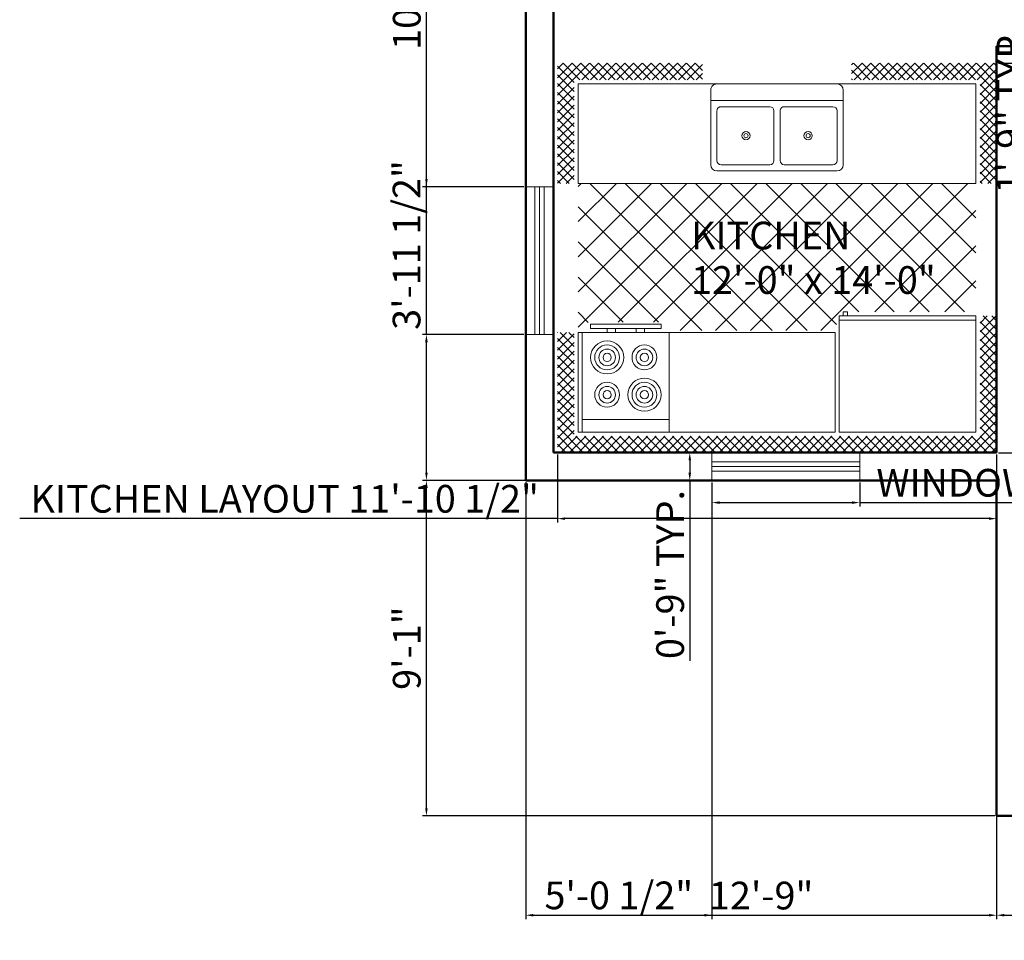
# Model space of a CAD drawing. Units: inches. Extents: x 2866 to 3545, y 873 to 1597.
# Tile 1 of 5: x 2866 to 3186, y 873 to 1172. Entities that reach past the tile are written whole.
import ezdxf

# ---------------------------------------------------------------- set-up
doc = ezdxf.new("R2010")
doc.units = ezdxf.units.IN
doc.layers.add('A-ANNO-DIMS', color=152, linetype='Continuous', lineweight=18, true_color=0x2776bb)
for name, color, linetype, lineweight in [('A-AREA-IDEN', 7, 'Continuous', 25), ('A-EQPM', 9, 'Continuous', 18), ('A-GLAZ', 4, 'Continuous', 18), ('A-WALL', 7, 'Continuous', 50)]:
    doc.layers.add(name, color=color, linetype=linetype, lineweight=lineweight)
doc.styles.get("Standard").update_dxf_attribs({"font": 'arial.ttf'})
doc.dimstyles.new('ISO-25', dxfattribs={"dimtxt": 9, "dimasz": 2.5, "dimexe": 1.25, "dimexo": 0.625, "dimtad": 1, "dimdec": 0, "dimlunit": 3, "dimtxsty": 'Standard', "dimcen": 4.5, "dimadec": 0, "dimazin": 0, "dimtfac": 1, "dimtdec": 0, "dimtmove": 0, "dimatfit": 3, "dimfxl": 1, "dimarcsym": 0})

# ---------------------------------------------------------------- blocks, each defined once
blk = doc.blocks.new('Kitchen Layout - 7 x 8 ft')
for p, q in [((-5, 81.32), (2.68, 89)), ((-5, 83.44), (0.56, 89)), ((-5, 85.56), (-1.56, 89)), ((-5, 87.68), (-3.68, 89)), ((-1, 84.97), (-5, 88.97)), ((1.09, 85), (-2.91, 89)), ((3.21, 85), (-0.79, 89)), ((0.81, 85), (4.81, 89)), ((5.34, 85), (1.34, 89)), ((2.93, 85), (6.93, 89)), ((7.46, 85), (3.46, 89)), ((5.05, 85), (9.05, 89)), ((9.58, 85), (5.58, 89)), ((7.17, 85), (11.17, 89)), ((11.7, 85), (7.7, 89)), ((9.29, 85), (13.29, 89)), ((13.82, 85), (9.82, 89)), ((11.41, 85), (15.41, 89)), ((15.94, 85), (11.94, 89)), ((13.53, 85), (17.53, 89)), ((18.06, 85), (14.06, 89)), ((15.65, 85), (19.65, 89)), ((20.18, 85), (16.18, 89)), ((17.78, 85), (21.78, 89)), ((22.31, 85), (18.31, 89)), ((19.9, 85), (23.9, 89)), ((24.43, 85), (20.43, 89)), ((22.02, 85), (26.02, 89)), ((26.55, 85), (22.55, 89)), ((24.14, 85), (28.14, 89)), ((28.67, 85), (24.67, 89)), ((26.26, 85), (30.26, 89)), ((30.79, 85), (26.79, 89)), ((28.38, 85), (32.38, 89)), ((32.91, 85), (28.91, 89)), ((30.5, 85), (34.5, 89)), ((35.03, 85), (31.03, 89)), ((32.63, 85), (36.63, 89)), ((37.16, 85), (33.16, 89)), ((34.75, 85), (38.75, 89)), ((39.28, 85), (35.28, 89)), ((36.87, 85), (40.87, 89)), ((41.4, 85), (37.4, 89)), ((38.99, 85), (42.99, 89)), ((43.52, 85), (39.52, 89)), ((41.11, 85), (45.11, 89)), ((45.64, 85), (41.64, 89)), ((43.23, 85), (47.23, 89)), ((47.76, 85), (43.76, 89)), ((45.35, 85), (49.35, 89)), ((49.88, 85), (45.88, 89)), ((47.47, 85), (51.47, 89)), ((52, 85), (48, 89)), ((49.6, 85), (53.6, 89)), ((54.13, 85), (50.13, 89)), ((51.72, 85), (55.72, 89)), ((56.25, 85), (52.25, 89)), ((53.84, 85), (57.84, 89)), ((58.37, 85), (54.37, 89)), ((55.96, 85), (59.96, 89)), ((60.49, 85), (56.49, 89)), ((58.08, 85), (62.08, 89)), ((62.61, 85), (58.61, 89)), ((60.2, 85), (64.2, 89)), ((64.73, 85), (60.73, 89)), ((62.32, 85), (66.32, 89)), ((66.85, 85), (62.85, 89)), ((64.45, 85), (68.45, 89)), ((68.97, 85), (64.97, 89)), ((66.57, 85), (70.57, 89)), ((71.1, 85), (67.1, 89)), ((68.69, 85), (72.69, 89)), ((73.22, 85), (69.22, 89)), ((70.81, 85), (74.81, 89)), ((75.34, 85), (71.34, 89)), ((72.93, 85), (76.93, 89)), ((77.46, 85), (73.46, 89)), ((75.05, 85), (79.05, 89)), ((79.58, 85), (75.58, 89)), ((77.17, 85), (81.17, 89)), ((81.7, 85), (77.7, 89)), ((79.29, 85), (83.29, 89)), ((83.82, 85), (79.82, 89)), ((81.42, 85), (85.42, 89)), ((85.95, 85), (81.95, 89)), ((83.54, 85), (87.54, 89)), ((88.07, 85), (84.07, 89)), ((85.66, 85), (89.66, 89)), ((90.19, 85), (86.19, 89)), ((87.78, 85), (91.78, 89)), ((92.31, 85), (88.31, 89)), ((89.9, 85), (93.9, 89)), ((94.43, 85), (90.43, 89)), ((92.02, 85), (96.02, 89)), ((96.55, 85), (92.55, 89)), ((94.14, 85), (98.14, 89)), ((101, 82.67), (94.67, 89)), ((96.27, 85), (100.27, 89)), ((101, 84.79), (96.79, 89)), ((101, 86.92), (98.92, 89)), ((-1, 82.85), (-5, 86.85)), ((97, 83.61), (101, 87.61)), ((-1, 80.73), (-5, 84.73)), ((-5, 79.19), (-1, 83.19)), ((34, 84), (96, 84)), ((34, 60), (34, 84)), ((96, 84), (96, 60)), ((97, 81.49), (101, 85.49)), ((101, 80.55), (97, 84.55)), ((97, 79.37), (101, 83.37)), ((-1, 78.61), (-5, 82.61)), ((-5, 77.07), (-1, 81.07)), ((74, 81), (95, 81)), ((101, 78.43), (97, 82.43)), ((97, 77.25), (101, 81.25)), ((-1, 76.49), (-5, 80.49)), ((-5, 74.95), (-1, 78.95)), ((101, 76.31), (97, 80.31)), ((97, 75.13), (101, 79.13)), ((-1, 74.36), (-5, 78.36)), ((-5, 72.83), (-1, 76.83)), ((-1, 72.24), (-5, 76.24)), ((101, 74.19), (97, 78.19)), ((97, 73.01), (101, 77.01)), ((101, 72.07), (97, 76.07)), ((-5, 70.71), (-1, 74.71)), ((-1, 70.12), (-5, 74.12)), ((97, 70.89), (101, 74.89)), ((101, 69.95), (97, 73.95)), ((-5, 68.59), (-1, 72.59)), ((-1, 68), (-5, 72)), ((97, 68.76), (101, 72.76)), ((101, 67.82), (97, 71.82)), ((-5, 66.47), (-1, 70.47)), ((-1, 65.88), (-5, 69.88)), ((97, 66.64), (101, 70.64)), ((101, 65.7), (97, 69.7)), ((-5, 64.35), (-1, 68.35)), ((-1, 63.76), (-5, 67.76)), ((97, 64.52), (101, 68.52)), ((101, 63.58), (97, 67.58)), ((-5, 62.22), (-1, 66.22)), ((-1, 61.64), (-5, 65.64)), ((97, 62.4), (101, 66.4)), ((101, 61.46), (97, 65.46)), ((97, 60.28), (101, 64.28)), ((-5, 60.1), (-1, 64.1)), ((-1, 59.52), (-5, 63.52)), ((-5, 57.98), (-1, 61.98)), ((100.34, 60), (97, 63.34)), ((98.84, 60), (101, 62.16)), ((-1, 57.39), (-5, 61.39)), ((-4.86, 56), (-1, 59.86)), ((10.4, 24), (45.9, 59.5)), ((18.88, 24), (54.38, 59.5)), ((27.37, 24), (62.87, 59.5)), ((33.03, 55.11), (37.41, 59.5)), ((96, 60), (34, 60)), ((35.85, 24), (71.35, 59.5)), ((76.2, 24), (40.7, 59.5)), ((84.68, 24), (49.18, 59.5)), ((93.17, 24), (57.67, 59.5)), ((96, 29.65), (66.15, 59.5)), ((80, 60), (80, 59)), ((82, 59), (82, 60)), ((87, 59), (87, 60)), ((89, 60), (89, 59)), ((98.22, 60), (97, 61.22)), ((100.96, 60), (101, 60.04)), ((-1.73, 56), (-5, 59.27)), ((-3.85, 56), (-5, 57.15)), ((-2.74, 56), (-1, 57.74)), ((67.71, 24), (33.68, 58.04)), ((44.34, 24), (77.84, 57.5)), ((52.82, 24), (86.32, 57.5)), ((61.31, 24), (96, 58.69)), ((96, 38.14), (76.64, 57.5)), ((96, 46.63), (85.13, 57.5)), ((96, 55.11), (93.57, 57.54)), ((0, 57), (33, 57)), ((0, 30.57), (24.43, 55)), ((0, 39.06), (15.94, 55)), ((0, 47.54), (7.46, 55)), ((1.91, 24), (32.91, 55)), ((33.77, 24), (2.77, 55)), ((42.26, 24), (11.26, 55)), ((50.74, 24), (19.74, 55)), ((59.23, 24), (28.23, 55)), ((31, 55), (31, 56)), ((32, 55), (31, 55)), ((32, 56), (32, 55)), ((69.79, 24), (96, 50.21)), ((25.29, 24), (0, 49.29)), ((16.8, 24), (0, 40.8)), ((78.28, 24), (96, 41.72)), ((8.32, 24), (0, 32.32)), ((86.76, 24), (96, 33.24)), ((-5, 21.92), (-2.92, 24)), ((-5, 19.8), (-1, 23.8)), ((-1, 21.33), (-3.67, 24)), ((-1, 23.45), (-1.55, 24)), ((0, 24), (96, 24)), ((0, 0), (0, 24)), ((95.25, 24), (96, 24.75)), ((96, 24), (96, 0)), ((97, 22.1), (98.9, 24)), ((97, 19.97), (101, 23.97)), ((101, 21.16), (98.16, 24)), ((101, 23.28), (100.28, 24)), ((-1, 19.21), (-5, 23.21)), ((-5, 17.68), (-1, 21.68)), ((101, 19.03), (97, 23.03)), ((97, 17.85), (101, 21.85)), ((-1, 17.09), (-5, 21.09)), ((-5, 15.55), (-1, 19.55)), ((101, 16.91), (97, 20.91)), ((97, 15.73), (101, 19.73)), ((-1, 14.97), (-5, 18.97)), ((-5, 13.43), (-1, 17.43)), ((-1, 12.85), (-5, 16.85)), ((47.25, 6.5), (47.25, 18.5)), ((48.75, 18.5), (48.75, 6.5)), ((101, 14.79), (97, 18.79)), ((97, 13.61), (101, 17.61)), ((101, 12.67), (97, 16.67)), ((-5, 11.31), (-1, 15.31)), ((-1, 10.73), (-5, 14.73)), ((97, 11.49), (101, 15.49)), ((101, 10.55), (97, 14.55)), ((-5, 9.19), (-1, 13.19)), ((-1, 8.6), (-5, 12.6)), ((97, 9.37), (101, 13.37)), ((101, 8.43), (97, 12.43)), ((-5, 7.07), (-1, 11.07)), ((-1, 6.48), (-5, 10.48)), ((97, 7.25), (101, 11.25)), ((101, 6.31), (97, 10.31)), ((-5, 4.95), (-1, 8.95)), ((-1, 4.36), (-5, 8.36)), ((97, 5.12), (101, 9.12)), ((101, 4.18), (97, 8.18)), ((-5, 2.83), (-1, 6.83)), ((-1, 2.24), (-5, 6.24)), ((97, 3), (101, 7)), ((101, 2.06), (97, 6.06)), ((97, 0.88), (101, 4.88)), ((-5, 0.71), (-1, 4.71)), ((-1, 0.12), (-5, 4.12)), ((-5, -1.42), (-1, 2.58)), ((64, 4), (32, 4)), ((93.24, -5), (101, 2.76)), ((101, -0.06), (97, 3.94)), ((2, -5), (-5, 2)), ((-5, -3.54), (-1, 0.46)), ((96, 0), (0, 0)), ((95.36, -5), (101, 0.64)), ((101, -2.18), (97, 1.82)), ((-0.12, -5), (-5, -0.12)), ((-2.25, -5), (-5, -2.25)), ((-4.34, -5), (-0.34, -1)), ((-2.22, -5), (1.78, -1)), ((-0.1, -5), (3.9, -1)), ((4.12, -5), (0.12, -1)), ((2.02, -5), (6.02, -1)), ((6.24, -5), (2.24, -1)), ((4.14, -5), (8.14, -1)), ((8.36, -5), (4.36, -1)), ((6.27, -5), (10.27, -1)), ((10.48, -5), (6.48, -1)), ((8.39, -5), (12.39, -1)), ((12.6, -5), (8.6, -1)), ((10.51, -5), (14.51, -1)), ((14.73, -5), (10.73, -1)), ((12.63, -5), (16.63, -1)), ((16.85, -5), (12.85, -1)), ((14.75, -5), (18.75, -1)), ((18.97, -5), (14.97, -1)), ((16.87, -5), (20.87, -1)), ((21.09, -5), (17.09, -1)), ((18.99, -5), (22.99, -1)), ((23.21, -5), (19.21, -1)), ((21.11, -5), (25.11, -1)), ((25.33, -5), (21.33, -1)), ((23.24, -5), (27.24, -1)), ((27.45, -5), (23.45, -1)), ((25.36, -5), (29.36, -1)), ((29.57, -5), (25.57, -1)), ((30, -3.3), (27.7, -1)), ((30, -1.18), (29.82, -1)), ((66, -2.54), (67.54, -1)), ((66, -4.66), (69.66, -1)), ((69.88, -5), (66, -1.12)), ((67.78, -5), (71.78, -1)), ((72, -5), (68, -1)), ((69.9, -5), (73.9, -1)), ((74.12, -5), (70.12, -1)), ((72.03, -5), (76.03, -1)), ((76.24, -5), (72.24, -1)), ((74.15, -5), (78.15, -1)), ((78.36, -5), (74.36, -1)), ((76.27, -5), (80.27, -1)), ((80.49, -5), (76.49, -1)), ((78.39, -5), (82.39, -1)), ((82.61, -5), (78.61, -1)), ((80.51, -5), (84.51, -1)), ((84.73, -5), (80.73, -1)), ((82.63, -5), (86.63, -1)), ((86.85, -5), (82.85, -1)), ((84.75, -5), (88.75, -1)), ((88.97, -5), (84.97, -1)), ((86.88, -5), (90.88, -1)), ((91.09, -5), (87.09, -1)), ((89, -5), (93, -1)), ((93.21, -5), (89.21, -1)), ((91.12, -5), (95.12, -1)), ((95.34, -5), (91.34, -1)), ((97.46, -5), (93.46, -1)), ((99.58, -5), (95.58, -1)), ((101, -4.3), (97, -0.3)), ((97.48, -5), (101, -1.48)), ((-4.37, -5), (-5, -4.37)), ((27.48, -5), (30, -2.48)), ((29.6, -5), (30, -4.6)), ((67.76, -5), (66, -3.24)), ((99.6, -5), (101, -3.6))]:
    blk.add_line(p, q)
for points in [[(0, 56), (0, 84), (33, 84), (33, 56)], [(74, 60), (74, 84), (95, 84), (95, 60)], [(76, 58), (76, 59), (93, 59), (93, 58)]]:
    blk.add_lwpolyline(points, close=True)
for points in [[(32, 1.5), (32, 19.5)], [(33.5, 21), (62.5, 21)], [(34.5, 19.5), (46.25, 19.5)], [(49.75, 19.5), (61.5, 19.5)], [(64, 19.5), (64, 1.5)], [(33.5, 6.5), (33.5, 18.5)], [(62.5, 18.5), (62.5, 6.5)], [(46.25, 5.5), (34.5, 5.5)], [(61.5, 5.5), (49.75, 5.5)], [(62.5, 0), (33.5, 0)]]:
    blk.add_lwpolyline(points)
for centre, radius in [((80, 75), 4), ((80, 75), 3), ((80, 75), 2), ((89, 75), 3), ((89, 75), 2), ((80, 75), 1), ((89, 75), 1), ((80, 66), 3), ((89, 66), 4), ((89, 66), 3), ((80, 66), 2), ((80, 66), 1), ((89, 66), 2), ((89, 66), 1), ((40.5, 12.5), 1), ((40.5, 12.5), 0.5), ((55.5, 12.5), 1), ((55.5, 12.5), 0.5)]:
    blk.add_circle(centre, radius)
for centre, radius, start, end in [((33.5, 19.5), 1.5, 90, 180), ((34.5, 18.5), 1, 90, 180), ((46.25, 18.5), 1, 0, 90), ((49.75, 18.5), 1, 90, 180), ((61.5, 18.5), 1, 0, 90), ((62.5, 19.5), 1.5, 0, 90), ((34.5, 6.5), 1, 180, 270), ((46.25, 6.5), 1, 270, 0), ((49.75, 6.5), 1, 180, 270), ((61.5, 6.5), 1, 270, 0), ((33.5, 1.5), 1.5, 180, 270), ((62.5, 1.5), 1.5, 270, 0)]:
    blk.add_arc(centre, radius, start, end)
blk = doc.blocks.new('WIN-48IN')
for p, q in [((0, 0), (0, 48)), ((0, 48), (9, 48)), ((3, 0), (3, 48)), ((4.5, 0), (4.5, 48)), ((6, 0), (6, 48)), ((9, 48), (9, 0)), ((9, 0), (0, 0))]:
    blk.add_line(p, q)
blk = doc.blocks.new('*D27')
at = {"layer": 'A-ANNO-DIMS', "color": 0, "lineweight": -2, "transparency": 16777216}
for p, q in [((3090.55, 1022.03), (3090.55, 1014.2)), ((3138.55, 1022.03), (3138.55, 1014.2)), ((3093.05, 1015.45), (3136.05, 1015.45)), ((3138.55, 1015.45), (3256.19, 1015.45))]:
    blk.add_line(p, q, dxfattribs=at)
at = {"layer": 'A-ANNO-DIMS', "color": 0, "transparency": 16777216}
for points in [[(3093.05, 1015.87), (3093.05, 1015.04), (3090.55, 1015.45)], [(3136.05, 1015.87), (3136.05, 1015.04), (3138.55, 1015.45)]]:
    blk.add_solid(points, dxfattribs=at)
at = {"layer": 'Defpoints', "color": 0, "transparency": 16777216}
for p in [(3090.55, 1022.65), (3138.55, 1022.65), (3138.55, 1015.45)]:
    blk.add_point(p, dxfattribs=at)
at = {"layer": 'A-ANNO-DIMS', "color": 0, "transparency": 16777216, "insert": (3198.62, 1020.73), "char_height": 9, "attachment_point": 5}
blk.add_mtext('WINDOW 4\'-0" TYP.', dxfattribs=at)
blk = doc.blocks.new('*D28')
at = {"layer": 'A-ANNO-DIMS', "color": 0, "lineweight": -2, "transparency": 16777216}
for p, q in [((3089.93, 1031.65), (3082.1, 1031.65)), ((3083.35, 1029.15), (3083.35, 1025.15)), ((3089.93, 1022.65), (3082.1, 1022.65)), ((3083.35, 1022.65), (3083.35, 964.04))]:
    blk.add_line(p, q, dxfattribs=at)
at = {"layer": 'A-ANNO-DIMS', "color": 0, "transparency": 16777216}
for points in [[(3082.93, 1029.15), (3083.77, 1029.15), (3083.35, 1031.65)], [(3082.93, 1025.15), (3083.77, 1025.15), (3083.35, 1022.65)]]:
    blk.add_solid(points, dxfattribs=at)
at = {"layer": 'Defpoints', "color": 0, "transparency": 16777216}
for p in [(3090.55, 1031.65), (3083.35, 1022.65), (3090.55, 1022.65)]:
    blk.add_point(p, dxfattribs=at)
at = {"layer": 'A-ANNO-DIMS', "color": 0, "transparency": 16777216, "insert": (3078.13, 992.1), "char_height": 9, "attachment_point": 5, "rotation": 90}
blk.add_mtext('0\'-9" TYP.', dxfattribs=at)
blk = doc.blocks.new('*D44')
at = {"layer": 'A-ANNO-DIMS', "color": 0, "lineweight": -2, "transparency": 16777216}
for p, q in [((3193.89, 1113.19), (3193.89, 1170.95)), ((3196.42, 1113.19), (3192.64, 1113.19)), ((3193.89, 1094.69), (3193.89, 1110.69)), ((3196.42, 1092.19), (3192.64, 1092.19))]:
    blk.add_line(p, q, dxfattribs=at)
at = {"layer": 'A-ANNO-DIMS', "color": 0, "transparency": 16777216}
for points in [[(3193.48, 1110.69), (3194.31, 1110.69), (3193.89, 1113.19)], [(3193.48, 1094.69), (3194.31, 1094.69), (3193.89, 1092.19)]]:
    blk.add_solid(points, dxfattribs=at)
at = {"layer": 'Defpoints', "color": 0, "transparency": 16777216}
for p in [(3193.89, 1113.19), (3197.04, 1113.19), (3197.04, 1092.19)]:
    blk.add_point(p, dxfattribs=at)
at = {"layer": 'A-ANNO-DIMS', "color": 0, "transparency": 16777216, "insert": (3188.67, 1143.32), "char_height": 9, "attachment_point": 5, "rotation": 90}
blk.add_mtext('1\'-9" TYP.', dxfattribs=at)
blk = doc.blocks.new('*D45')
at = {"layer": 'A-ANNO-DIMS', "color": 0, "lineweight": -2, "transparency": 16777216}
for p, q in [((3040.36, 1031.03), (3040.36, 1009)), ((3183.04, 1031.03), (3183.04, 1009)), ((3040.36, 1010.25), (2865.65, 1010.25)), ((3180.54, 1010.25), (3042.86, 1010.25))]:
    blk.add_line(p, q, dxfattribs=at)
at = {"layer": 'A-ANNO-DIMS', "color": 0, "transparency": 16777216}
for points in [[(3042.86, 1010.67), (3042.86, 1009.83), (3040.36, 1010.25)], [(3180.54, 1010.67), (3180.54, 1009.83), (3183.04, 1010.25)]]:
    blk.add_solid(points, dxfattribs=at)
at = {"layer": 'Defpoints', "color": 0, "transparency": 16777216}
for p in [(3040.36, 1031.65), (3183.04, 1031.65), (3040.36, 1010.25)]:
    blk.add_point(p, dxfattribs=at)
at = {"layer": 'A-ANNO-DIMS', "color": 0, "transparency": 16777216, "insert": (2951.76, 1015.53), "char_height": 9, "attachment_point": 5}
blk.add_mtext('KITCHEN LAYOUT 11\'-10 1/2"', dxfattribs=at)
blk = doc.blocks.new('*D46')
at = {"layer": 'A-ANNO-DIMS', "color": 0, "lineweight": -2, "transparency": 16777216}
for p, q in [((3183.67, 1158.18), (3205.69, 1158.18)), ((3204.44, 1155.68), (3204.44, 1034.15)), ((3183.67, 1031.65), (3205.69, 1031.65))]:
    blk.add_line(p, q, dxfattribs=at)
at = {"layer": 'A-ANNO-DIMS', "color": 0, "transparency": 16777216}
for points in [[(3204.03, 1155.68), (3204.86, 1155.68), (3204.44, 1158.18)], [(3204.03, 1034.15), (3204.86, 1034.15), (3204.44, 1031.65)]]:
    blk.add_solid(points, dxfattribs=at)
at = {"layer": 'Defpoints', "color": 0, "transparency": 16777216}
for p in [(3183.04, 1158.18), (3183.04, 1031.65), (3204.44, 1031.65)]:
    blk.add_point(p, dxfattribs=at)
at = {"layer": 'A-ANNO-DIMS', "color": 0, "transparency": 16777216, "insert": (3199.17, 1094.92), "char_height": 9, "attachment_point": 5, "rotation": 90}
blk.add_mtext('10\'-6 1/2"', dxfattribs=at)
blk = doc.blocks.new('*D60')
at = {"layer": 'A-ANNO-DIMS', "color": 0, "lineweight": -2, "transparency": 16777216}
for p, q in [((3030.04, 1022.07), (3030.04, 880.19)), ((3183.04, 1022.07), (3183.04, 880.19)), ((3032.54, 881.44), (3180.54, 881.44))]:
    blk.add_line(p, q, dxfattribs=at)
at = {"layer": 'A-ANNO-DIMS', "color": 0, "transparency": 16777216}
for points in [[(3032.54, 881.86), (3032.54, 881.03), (3030.04, 881.44)], [(3180.54, 881.86), (3180.54, 881.03), (3183.04, 881.44)]]:
    blk.add_solid(points, dxfattribs=at)
at = {"layer": 'Defpoints', "color": 0, "transparency": 16777216}
for p in [(3030.04, 1022.69), (3183.04, 1022.69), (3183.04, 881.44)]:
    blk.add_point(p, dxfattribs=at)
at = {"layer": 'A-ANNO-DIMS', "color": 0, "transparency": 16777216, "insert": (3106.54, 886.66), "char_height": 9, "attachment_point": 5}
blk.add_mtext('12\'-9"', dxfattribs=at)
blk = doc.blocks.new('*D61')
at = {"layer": 'A-ANNO-DIMS', "color": 0, "lineweight": -2, "transparency": 16777216}
for p, q in [((3182.42, 1022.69), (2996.54, 1022.69)), ((2997.79, 916.19), (2997.79, 1020.19)), ((3182.42, 913.69), (2996.54, 913.69))]:
    blk.add_line(p, q, dxfattribs=at)
at = {"layer": 'A-ANNO-DIMS', "color": 0, "transparency": 16777216}
for points in [[(2997.38, 1020.19), (2998.21, 1020.19), (2997.79, 1022.69)], [(2997.38, 916.19), (2998.21, 916.19), (2997.79, 913.69)]]:
    blk.add_solid(points, dxfattribs=at)
at = {"layer": 'Defpoints', "color": 0, "transparency": 16777216}
for p in [(2997.79, 1022.69), (3183.04, 1022.69), (3183.04, 913.69)]:
    blk.add_point(p, dxfattribs=at)
at = {"layer": 'A-ANNO-DIMS', "color": 0, "transparency": 16777216, "insert": (2992.57, 968.19), "char_height": 9, "attachment_point": 5, "rotation": 90}
blk.add_mtext('9\'-1"', dxfattribs=at)
blk = doc.blocks.new('*D62')
at = {"layer": 'A-ANNO-DIMS', "color": 0, "lineweight": -2, "transparency": 16777216}
for p, q in [((3183.04, 913.07), (3183.04, 880.19)), ((3255.04, 913.07), (3255.04, 880.19)), ((3185.54, 881.44), (3252.54, 881.44))]:
    blk.add_line(p, q, dxfattribs=at)
at = {"layer": 'A-ANNO-DIMS', "color": 0, "transparency": 16777216}
for points in [[(3185.54, 881.86), (3185.54, 881.03), (3183.04, 881.44)], [(3252.54, 881.86), (3252.54, 881.03), (3255.04, 881.44)]]:
    blk.add_solid(points, dxfattribs=at)
at = {"layer": 'Defpoints', "color": 0, "transparency": 16777216}
for p in [(3183.04, 913.69), (3255.04, 913.69), (3255.04, 881.44)]:
    blk.add_point(p, dxfattribs=at)
at = {"layer": 'A-ANNO-DIMS', "color": 0, "transparency": 16777216, "insert": (3219.04, 886.66), "char_height": 9, "attachment_point": 5}
blk.add_mtext('6\'-0"', dxfattribs=at)
blk = doc.blocks.new('*D68')
at = {"layer": 'A-ANNO-DIMS', "color": 0, "lineweight": -2, "transparency": 16777216}
for p, q in [((2997.79, 1070.06), (2997.79, 1125.69)), ((3029.42, 1070.06), (2996.54, 1070.06)), ((2997.79, 1025.19), (2997.79, 1067.56)), ((3029.42, 1022.69), (2996.54, 1022.69))]:
    blk.add_line(p, q, dxfattribs=at)
at = {"layer": 'A-ANNO-DIMS', "color": 0, "transparency": 16777216}
for points in [[(2997.38, 1067.56), (2998.21, 1067.56), (2997.79, 1070.06)], [(2997.38, 1025.19), (2998.21, 1025.19), (2997.79, 1022.69)]]:
    blk.add_solid(points, dxfattribs=at)
at = {"layer": 'Defpoints', "color": 0, "transparency": 16777216}
for p in [(2997.79, 1070.06), (3030.04, 1070.06), (3030.04, 1022.69)]:
    blk.add_point(p, dxfattribs=at)
at = {"layer": 'A-ANNO-DIMS', "color": 0, "transparency": 16777216, "insert": (2992.51, 1099.13), "char_height": 9, "attachment_point": 5, "rotation": 90}
blk.add_mtext('3\'-11 1/2"', dxfattribs=at)
blk = doc.blocks.new('*D69')
at = {"layer": 'A-ANNO-DIMS', "color": 0, "lineweight": -2, "transparency": 16777216}
for p, q in [((3029.42, 1240.84), (2996.54, 1240.84)), ((2997.79, 1120.56), (2997.79, 1238.34)), ((3029.42, 1118.06), (2996.54, 1118.06))]:
    blk.add_line(p, q, dxfattribs=at)
at = {"layer": 'A-ANNO-DIMS', "color": 0, "transparency": 16777216}
for points in [[(2997.38, 1238.34), (2998.21, 1238.34), (2997.79, 1240.84)], [(2997.38, 1120.56), (2998.21, 1120.56), (2997.79, 1118.06)]]:
    blk.add_solid(points, dxfattribs=at)
at = {"layer": 'Defpoints', "color": 0, "transparency": 16777216}
for p in [(2997.79, 1240.84), (3030.04, 1240.84), (3030.04, 1118.06)]:
    blk.add_point(p, dxfattribs=at)
at = {"layer": 'A-ANNO-DIMS', "color": 0, "transparency": 16777216, "insert": (2992.57, 1179.45), "char_height": 9, "attachment_point": 5, "rotation": 90}
blk.add_mtext('10\'-3"', dxfattribs=at)
blk = doc.blocks.new('*D74')
at = {"layer": 'A-ANNO-DIMS', "color": 0, "lineweight": -2, "transparency": 16777216}
for p, q in [((3030.04, 1022.07), (3030.04, 880.19)), ((3090.55, 1022.03), (3090.55, 880.19)), ((3032.54, 881.44), (3088.05, 881.44))]:
    blk.add_line(p, q, dxfattribs=at)
at = {"layer": 'A-ANNO-DIMS', "color": 0, "transparency": 16777216}
for points in [[(3032.54, 881.86), (3032.54, 881.03), (3030.04, 881.44)], [(3088.05, 881.86), (3088.05, 881.03), (3090.55, 881.44)]]:
    blk.add_solid(points, dxfattribs=at)
at = {"layer": 'Defpoints', "color": 0, "transparency": 16777216}
for p in [(3030.04, 1022.69), (3090.55, 1022.65), (3090.55, 881.44)]:
    blk.add_point(p, dxfattribs=at)
at = {"layer": 'A-ANNO-DIMS', "color": 0, "transparency": 16777216, "insert": (3060.3, 886.72), "char_height": 9, "attachment_point": 5}
blk.add_mtext('5\'-0 1/2"', dxfattribs=at)

msp = doc.modelspace()

# ---------------------------------------------------------------- linework, layer by layer
at = {"layer": 'A-WALL'}
for p, q in [((3030.04, 1523.69), (3030.04, 1022.69)), ((3039.04, 1199.69), (3039.04, 1031.69)), ((3183.04, 1163.69), (3183.04, 1031.69)), ((3183.04, 1163.69), (3188.04, 1163.69)), ((3039.04, 1031.69), (3183.04, 1031.69)), ((3030.04, 1022.69), (3183.04, 1022.69)), ((3183.04, 1022.69), (3183.04, 913.69)), ((3183.04, 913.69), (3255.04, 913.69))]:
    msp.add_line(p, q, dxfattribs=at)

# ---------------------------------------------------------------- block references
at = {"layer": 'A-EQPM', "xscale": 1.346053094351419, "yscale": 1.346053094351419, "zscale": 1.346053094351419, "rotation": 180}
msp.add_blockref('Kitchen Layout - 7 x 8 ft', (3176.31, 1151.45), dxfattribs=at)
at = {"layer": 'A-GLAZ'}
msp.add_blockref('WIN-48IN', (3030.04, 1070.06), dxfattribs=at)
at = {"layer": 'A-GLAZ', "rotation": 269.9999999999995}
msp.add_blockref('WIN-48IN', (3090.55, 1031.65), dxfattribs=at)

# ---------------------------------------------------------------- texts
at = {"layer": 'A-AREA-IDEN'}
for s, p in [('KITCHEN', (3083.77, 1097.7)), ('12\'-0" x 14\'-0"', (3083.77, 1083.25))]:
    msp.add_text(s, height=9, dxfattribs=at).set_placement(p)

# ---------------------------------------------------------------- dimensions: what is measured, and where the dimension line sits
at = {"layer": 'A-ANNO-DIMS'}
for base, p1, p2, angle, picture, middle in [((2997.79, 1240.84), (3030.04, 1118.06), (3030.04, 1240.84), 90, '*D69', (2992.57, 1179.45)), ((3204.44, 1031.65), (3183.04, 1158.18), (3183.04, 1031.65), 270, '*D46', (3199.17, 1094.92)), ((2997.79, 1070.06), (3030.04, 1022.69), (3030.04, 1070.06), 90, '*D68', (2992.51, 1099.13)), ((2997.79, 1022.69), (3183.04, 913.69), (3183.04, 1022.69), 90, '*D61', (2992.57, 968.19))]:
    dim = msp.add_linear_dim(base=base, p1=p1, p2=p2, angle=angle, dimstyle='ISO-25', override={"dimdec": 1, "dimlfac": 1, "dimrnd": 0, "dimzin": 1, "dimdsep": 46, "dimlunit": 4, "dimfrac": 2}, dxfattribs=at)
    dim.commit()
    dim.dimension.update_dxf_attribs({"geometry": picture, "text_midpoint": middle})
for base, p1, p2, angle, text, picture, middle in [((3193.89, 1113.19), (3197.04, 1092.19), (3197.04, 1113.19), 90, '<> TYP.', '*D44', (3188.67, 1143.32)), ((3040.36, 1010.25), (3183.04, 1031.65), (3040.36, 1031.65), 180, 'KITCHEN LAYOUT <>', '*D45', (2951.76, 1015.53)), ((3083.35, 1022.65), (3090.55, 1031.65), (3090.55, 1022.65), 270, '<> TYP.', '*D28', (3078.13, 992.1))]:
    dim = msp.add_linear_dim(base=base, p1=p1, p2=p2, angle=angle, text=text, dimstyle='ISO-25', override={"dimdec": 1, "dimlfac": 1, "dimrnd": 0, "dimzin": 1, "dimdsep": 46, "dimlunit": 4, "dimfrac": 2}, dxfattribs=at)
    dim.commit()
    dim.dimension.update_dxf_attribs({"geometry": picture, "text_midpoint": middle})
dim = msp.add_linear_dim(base=(3138.55, 1015.45), p1=(3090.55, 1022.65), p2=(3138.55, 1022.65), text='WINDOW <> TYP.', dimstyle='ISO-25', override={"dimdec": 1, "dimlfac": 1, "dimrnd": 0, "dimzin": 1, "dimdsep": 46, "dimlunit": 4, "dimfrac": 2}, dxfattribs=at)
dim.commit()
dim.dimension.update_dxf_attribs({"geometry": '*D27', "text_midpoint": (3198.62, 1020.73)})
for base, p1, p2, picture, middle in [((3183.04, 881.44), (3030.04, 1022.69), (3183.04, 1022.69), '*D60', (3106.54, 886.66)), ((3090.55, 881.44), (3030.04, 1022.69), (3090.55, 1022.65), '*D74', (3060.3, 886.72)), ((3255.04, 881.44), (3183.04, 913.69), (3255.04, 913.69), '*D62', (3219.04, 886.66))]:
    dim = msp.add_linear_dim(base=base, p1=p1, p2=p2, dimstyle='ISO-25', override={"dimdec": 1, "dimlfac": 1, "dimrnd": 0, "dimzin": 1, "dimdsep": 46, "dimlunit": 4, "dimfrac": 2}, dxfattribs=at)
    dim.commit()
    dim.dimension.update_dxf_attribs({"geometry": picture, "text_midpoint": middle})

doc.saveas('drawing.dxf')
